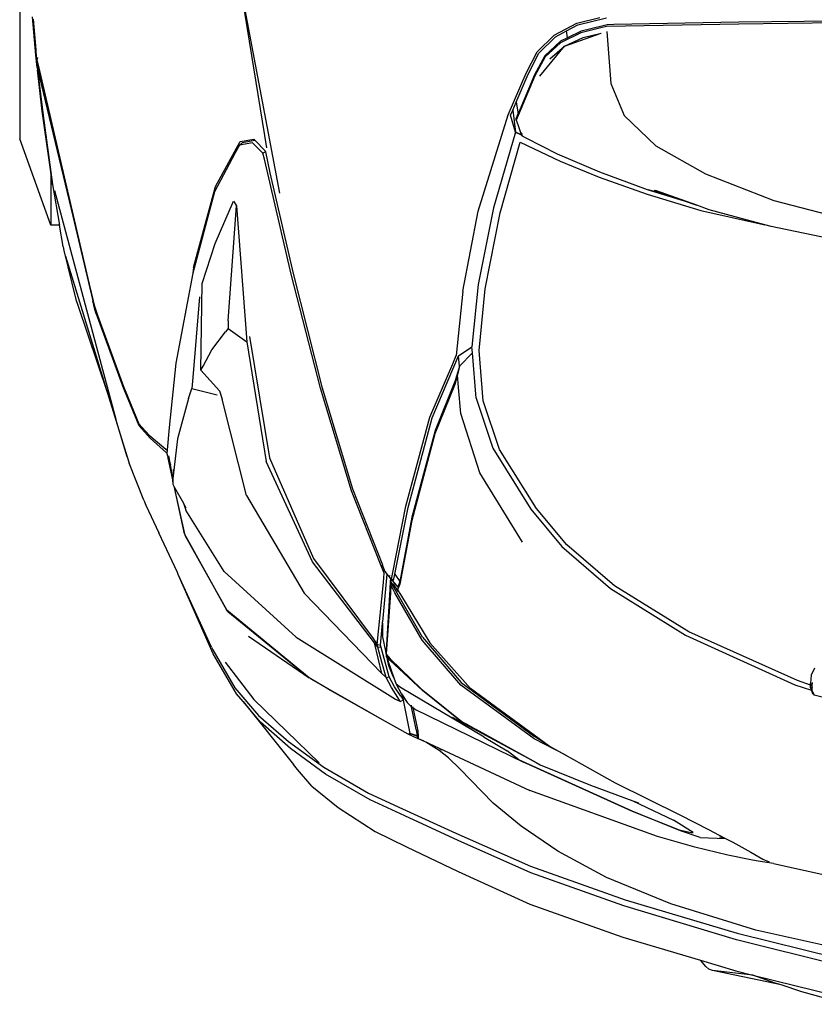
# Model space of a CAD drawing. Units: inches. Extents: x -4737294 to -4736756, y 1716389 to 1717040.
# Tile 3 of 25: x -4737188 to -4737168, y 1716466 to 1716491. Entities that reach past the tile are written whole.
import ezdxf

# ---------------------------------------------------------------- set-up
doc = ezdxf.new("R2010")
doc.units = ezdxf.units.IN
doc.header["$MEASUREMENT"] = 0
doc.layers.add('A-EQPM-VEHI', color=250, linetype='Continuous', lineweight=13)
doc.layers.add('Edges', color=250, linetype='Continuous')

# ---------------------------------------------------------------- blocks, each defined once
blk = doc.blocks.new('Nissan Qashqai pl')
at = {"layer": 'Edges'}
for p, q in [((11.05947, 11.55994), (11.06074, 11.45082)), ((11.06059, 11.56009), (11.06182, 11.4509)), ((11.6016, 11.52761), (11.58664, 11.46068)), ((11.58843, 11.44985), (11.60765, 11.5276)), ((11.61178, 11.52762), (11.59225, 11.44945)), ((11.61272, 11.45895), (11.62966, 11.52759)), ((11.16395, 11.47112), (11.17758, 11.52307)), ((11.45032, 11.49453), (11.45676, 11.51971)), ((11.18773, 11.51111), (11.17906, 11.46956)), ((11.54814, 11.47101), (11.55707, 11.51104)), ((11.62771, 11.50627), (11.62241, 11.48743)), ((11.435, 11.49469), (11.43896, 11.49272)), ((11.44507, 11.49341), (11.44316, 11.49351)), ((11.44373, 11.49245), (11.44491, 11.49291)), ((11.44453, 11.48334), (11.44778, 11.49299)), ((11.44491, 11.49291), (11.44474, 11.49242)), ((11.44507, 11.49341), (11.44491, 11.49291)), ((11.44491, 11.49291), (11.44606, 11.49335)), ((11.44606, 11.49335), (11.44507, 11.49341)), ((11.44786, 11.49325), (11.44606, 11.49335)), ((11.44786, 11.49325), (11.4462, 11.49239)), ((11.44778, 11.49299), (11.4462, 11.49239)), ((11.45018, 11.49392), (11.44778, 11.49299)), ((11.44794, 11.49325), (11.44786, 11.49325)), ((11.45032, 11.49453), (11.44794, 11.49325)), ((11.45018, 11.49392), (11.45032, 11.49453)), ((11.43896, 11.49272), (11.44373, 11.49245)), ((11.44474, 11.49242), (11.44218, 11.48476)), ((11.44474, 11.49242), (11.44373, 11.49245)), ((11.4462, 11.49239), (11.44474, 11.49242)), ((11.62241, 11.48743), (11.61848, 11.47528)), ((11.44218, 11.48476), (11.41383, 11.42186)), ((11.41588, 11.41997), (11.44453, 11.48334)), ((11.14869, 11.43161), (11.16395, 11.47112)), ((11.54814, 11.47101), (11.54666, 11.46197)), ((11.61848, 11.47528), (11.61008, 11.43562)), ((11.61742, 11.47198), (11.61272, 11.45895)), ((11.61848, 11.47528), (11.61742, 11.47198)), ((11.17808, 11.46592), (11.1694, 11.43374)), ((11.1699, 11.42889), (11.17797, 11.4652)), ((11.17797, 11.4652), (11.17808, 11.46592)), ((11.17906, 11.46956), (11.17808, 11.46592)), ((11.54162, 11.45783), (11.54554, 11.46484)), ((11.54554, 11.46484), (11.54721, 11.46841)), ((11.54611, 11.45874), (11.54336, 11.44449)), ((11.54666, 11.46197), (11.54611, 11.45874)), ((11.58664, 11.46068), (11.57152, 11.41151)), ((11.61272, 11.45895), (11.61008, 11.43562)), ((11.61028, 11.44915), (11.61272, 11.45895)), ((11.53572, 11.44731), (11.54162, 11.45783)), ((11.06074, 11.45082), (11.06214, 11.37845)), ((11.06182, 11.4509), (11.06324, 11.37414)), ((11.53354, 11.44315), (11.53572, 11.44731)), ((11.56912, 11.38501), (11.58843, 11.44985)), ((11.59225, 11.44945), (11.57263, 11.38419)), ((11.60419, 11.42861), (11.61028, 11.44915)), ((11.52833, 11.43321), (11.53335, 11.4428)), ((11.53261, 11.43965), (11.5333, 11.44225)), ((11.53313, 11.42848), (11.53354, 11.44315)), ((11.5333, 11.44225), (11.53335, 11.4428)), ((11.53335, 11.4428), (11.53354, 11.44315)), ((11.54336, 11.44449), (11.53855, 11.42543)), ((11.1323, 11.40268), (11.14869, 11.43161)), ((11.1694, 11.43374), (11.1668, 11.42651)), ((11.5202, 11.41712), (11.52833, 11.43321)), ((11.60772, 11.43162), (11.60419, 11.42861)), ((11.60938, 11.43347), (11.60772, 11.43162)), ((11.61008, 11.43562), (11.60938, 11.43347)), ((11.1668, 11.42651), (11.1582, 11.40259)), ((11.16047, 11.39766), (11.1699, 11.42889)), ((11.16426, 11.41918), (11.1668, 11.42651)), ((11.53313, 11.42848), (11.52922, 11.417)), ((11.53855, 11.42543), (11.53253, 11.4038)), ((11.59084, 11.38361), (11.60419, 11.42861)), ((11.15764, 11.39828), (11.16426, 11.41918)), ((11.15766, 11.39771), (11.16426, 11.41918)), ((11.16426, 11.41918), (11.15826, 11.40186)), ((11.41383, 11.42186), (11.38718, 11.37878)), ((11.38877, 11.37638), (11.41588, 11.41997)), ((11.53009, 11.42439), (11.52299, 11.41307)), ((11.52855, 11.41625), (11.53022, 11.42324)), ((11.53022, 11.42324), (11.53009, 11.42439)), ((11.50131, 11.37908), (11.5202, 11.41712)), ((11.5118, 11.38938), (11.52299, 11.41307)), ((11.52922, 11.417), (11.51787, 11.38901)), ((11.51787, 11.38901), (11.52855, 11.41625)), ((11.57152, 11.41151), (11.55624, 11.37411)), ((11.11477, 11.38434), (11.1323, 11.40268)), ((11.53253, 11.4038), (11.50574, 11.32965)), ((11.14751, 11.37001), (11.15766, 11.39771)), ((11.15051, 11.36998), (11.16047, 11.39766)), ((11.5118, 11.38938), (11.51304, 11.39274)), ((11.51787, 11.38901), (11.48801, 11.32337)), ((11.49005, 11.3275), (11.51787, 11.38901)), ((11.50277, 11.36495), (11.5118, 11.38938)), ((11.54963, 11.33002), (11.56912, 11.38501)), ((11.09618, 11.37663), (11.11477, 11.38434)), ((11.48518, 11.35017), (11.50131, 11.37908)), ((11.57263, 11.38419), (11.5535, 11.33028)), ((11.57164, 11.32969), (11.59084, 11.38361)), ((11.06236, 11.3576), (11.05822, 11.37418)), ((11.06214, 11.37845), (11.06222, 11.37449)), ((11.06222, 11.37449), (11.06303, 11.37135)), ((11.06324, 11.37414), (11.06408, 11.37085)), ((11.06624, 11.37435), (11.09618, 11.37663)), ((11.38718, 11.37878), (11.3635, 11.35125)), ((11.36451, 11.34835), (11.38877, 11.37638)), ((11.55624, 11.37411), (11.54097, 11.34593)), ((11.06139, 11.35691), (11.05807, 11.37037)), ((11.06303, 11.37135), (11.06594, 11.3594)), ((11.06408, 11.37085), (11.06692, 11.35921)), ((11.06961, 11.36056), (11.0671, 11.37109)), ((11.07472, 11.34981), (11.0671, 11.37109)), ((11.13692, 11.34555), (11.14751, 11.37001)), ((11.14123, 11.34726), (11.15051, 11.36998)), ((11.49086, 11.33567), (11.50277, 11.36495)), ((11.06818, 11.34377), (11.06139, 11.35691)), ((11.06584, 11.35092), (11.06236, 11.3576)), ((11.06594, 11.3594), (11.06978, 11.35164)), ((11.06692, 11.35921), (11.0727, 11.34754)), ((11.07472, 11.34981), (11.06961, 11.36056)), ((11.06978, 11.35164), (11.06584, 11.35092)), ((11.06918, 11.34452), (11.06584, 11.35092)), ((11.06978, 11.35164), (11.07183, 11.3475)), ((11.3635, 11.35125), (11.34251, 11.3336)), ((11.07183, 11.3475), (11.08018, 11.33842)), ((11.0727, 11.34754), (11.0809, 11.33858)), ((11.08206, 11.34125), (11.07472, 11.34981)), ((11.092, 11.33548), (11.07472, 11.34981)), ((11.12767, 11.32749), (11.13692, 11.34555)), ((11.13017, 11.32416), (11.14123, 11.34726)), ((11.34283, 11.33026), (11.36451, 11.34835)), ((11.48518, 11.35017), (11.4758, 11.33232)), ((11.48012, 11.34111), (11.48518, 11.35017)), ((11.54097, 11.34593), (11.52646, 11.32473)), ((11.07787, 11.3339), (11.06818, 11.34377)), ((11.07866, 11.33492), (11.06918, 11.34452)), ((11.48005, 11.341), (11.44669, 11.29536)), ((11.47876, 11.33901), (11.47454, 11.33252)), ((11.47876, 11.33901), (11.48005, 11.341)), ((11.48005, 11.341), (11.48012, 11.34111)), ((11.09022, 11.32753), (11.07787, 11.3339)), ((11.09081, 11.32882), (11.07866, 11.33492)), ((11.08018, 11.33842), (11.09121, 11.33249)), ((11.0809, 11.33858), (11.09174, 11.33271)), ((11.34251, 11.3336), (11.3082, 11.31215)), ((11.46332, 11.28473), (11.48966, 11.33337)), ((11.47038, 11.29841), (11.49086, 11.33567)), ((11.47038, 11.29841), (11.48966, 11.33337)), ((11.48966, 11.33337), (11.49086, 11.33567)), ((11.11439, 11.31711), (11.09022, 11.32753)), ((11.10704, 11.32181), (11.09081, 11.32882)), ((11.09121, 11.33249), (11.1138, 11.3229)), ((11.09174, 11.33271), (11.11486, 11.323)), ((11.12645, 11.32495), (11.12767, 11.32749)), ((11.30757, 11.30833), (11.34283, 11.33026)), ((11.44331, 11.28988), (11.47454, 11.33252)), ((11.4758, 11.33232), (11.44474, 11.28965)), ((11.48133, 11.27727), (11.50574, 11.32965)), ((11.48983, 11.32694), (11.49005, 11.3275)), ((11.53062, 11.28691), (11.54963, 11.33002)), ((11.5535, 11.33028), (11.53487, 11.28826)), ((11.55274, 11.28821), (11.57164, 11.32969)), ((11.10704, 11.32181), (11.1138, 11.3229)), ((11.11164, 11.31982), (11.10704, 11.32181)), ((11.1138, 11.3229), (11.11393, 11.32284)), ((11.11393, 11.32284), (11.1164, 11.32172)), ((11.11486, 11.323), (11.1172, 11.32196)), ((11.1164, 11.32172), (11.1172, 11.32196)), ((11.11744, 11.32189), (11.1164, 11.32172)), ((11.1172, 11.32196), (11.11744, 11.32189)), ((11.11744, 11.32189), (11.11997, 11.32267)), ((11.11997, 11.32267), (11.12459, 11.32429)), ((11.12604, 11.32481), (11.1244, 11.32146)), ((11.1244, 11.32146), (11.12591, 11.32476)), ((11.12459, 11.32429), (11.12591, 11.32476)), ((11.12466, 11.32442), (11.12595, 11.32486)), ((11.12478, 11.32467), (11.12595, 11.32486)), ((11.12595, 11.32486), (11.1251, 11.3253)), ((11.12591, 11.32476), (11.12595, 11.32486)), ((11.12591, 11.32476), (11.12604, 11.32481)), ((11.12595, 11.32486), (11.12626, 11.32554)), ((11.12595, 11.32486), (11.12607, 11.32488)), ((11.12604, 11.32481), (11.12645, 11.32495)), ((11.12607, 11.32488), (11.12604, 11.32481)), ((11.12631, 11.32537), (11.12607, 11.32488)), ((11.12607, 11.32488), (11.12645, 11.32495)), ((11.17121, 11.31245), (11.13017, 11.32416)), ((11.36192, 11.32544), (11.32179, 11.30083)), ((11.45883, 11.26345), (11.48954, 11.32636)), ((11.48801, 11.32337), (11.48281, 11.31653)), ((11.48983, 11.32694), (11.48954, 11.32636)), ((11.52646, 11.32473), (11.51313, 11.30854)), ((11.11164, 11.31982), (11.1244, 11.32146)), ((11.11467, 11.31851), (11.11164, 11.31982)), ((11.17021, 11.29978), (11.11439, 11.31711)), ((11.1244, 11.32146), (11.11467, 11.31851)), ((11.1244, 11.32146), (11.16836, 11.30873)), ((11.47499, 11.30324), (11.48281, 11.31653)), ((11.21523, 11.3038), (11.17121, 11.31245)), ((11.3082, 11.31215), (11.28005, 11.30276)), ((11.16836, 11.30873), (11.21271, 11.29983)), ((11.27848, 11.29865), (11.30757, 11.30833)), ((11.51313, 11.30854), (11.49329, 11.28912)), ((11.21656, 11.2908), (11.17021, 11.29978)), ((11.21271, 11.29983), (11.24875, 11.29618)), ((11.2509, 11.3003), (11.21523, 11.3038)), ((11.28005, 11.30276), (11.2509, 11.3003)), ((11.32179, 11.30083), (11.28736, 11.28974)), ((11.47499, 11.30324), (11.4462, 11.25482)), ((11.25238, 11.29648), (11.24875, 11.29618)), ((11.2541, 11.28846), (11.24875, 11.29618)), ((11.27848, 11.29865), (11.25238, 11.29648)), ((11.25238, 11.29648), (11.25993, 11.28891)), ((11.42028, 11.27173), (11.44669, 11.29536)), ((11.46746, 11.29312), (11.47026, 11.29821)), ((11.47026, 11.29821), (11.47038, 11.29841)), ((11.21656, 11.2908), (11.25377, 11.28706)), ((11.25993, 11.28891), (11.2541, 11.28846)), ((11.29, 11.2731), (11.2541, 11.28846)), ((11.25993, 11.28891), (11.25999, 11.28889)), ((11.25999, 11.28889), (11.26503, 11.28789)), ((11.25999, 11.28889), (11.26771, 11.28668)), ((11.27242, 11.28847), (11.26503, 11.28789)), ((11.26503, 11.28789), (11.27055, 11.28622)), ((11.28736, 11.28974), (11.27242, 11.28847)), ((11.41708, 11.26758), (11.44331, 11.28988)), ((11.44474, 11.28965), (11.41866, 11.26734)), ((11.44691, 11.26684), (11.46587, 11.29022)), ((11.46538, 11.28932), (11.44788, 11.2676)), ((11.46538, 11.28932), (11.46587, 11.29022)), ((11.46587, 11.29022), (11.46737, 11.29293)), ((11.46746, 11.29312), (11.46737, 11.29293)), ((11.49329, 11.28912), (11.48692, 11.28262)), ((11.53487, 11.28826), (11.52058, 11.25724)), ((11.53843, 11.2583), (11.55274, 11.28821)), ((11.25857, 11.28503), (11.25377, 11.28706)), ((11.28951, 11.27177), (11.25857, 11.28503)), ((11.26771, 11.28668), (11.26785, 11.28663)), ((11.26785, 11.28663), (11.29721, 11.27493)), ((11.27055, 11.28622), (11.29928, 11.27468)), ((11.48692, 11.28262), (11.48256, 11.27724)), ((11.51652, 11.25601), (11.53062, 11.28691)), ((11.47707, 11.26812), (11.48133, 11.27727)), ((11.48256, 11.27724), (11.47783, 11.26953)), ((11.48133, 11.27727), (11.48217, 11.27864)), ((11.3411, 11.25789), (11.28951, 11.27177)), ((11.34188, 11.25916), (11.29, 11.2731)), ((11.29721, 11.27493), (11.34742, 11.26142)), ((11.29928, 11.27468), (11.34932, 11.2614)), ((11.39234, 11.25471), (11.42028, 11.27173)), ((11.41708, 11.26758), (11.38507, 11.24911)), ((11.41866, 11.26734), (11.3914, 11.25156)), ((11.42958, 11.2488), (11.44691, 11.26684)), ((11.44788, 11.2676), (11.43028, 11.24852)), ((11.46049, 11.26254), (11.47129, 11.26473)), ((11.47129, 11.26473), (11.47442, 11.26498)), ((11.47585, 11.26509), (11.47322, 11.2592)), ((11.47442, 11.26498), (11.47433, 11.26475)), ((11.47442, 11.26498), (11.47446, 11.26498)), ((11.47445, 11.26477), (11.47446, 11.26498)), ((11.47446, 11.26498), (11.47482, 11.26501)), ((11.47585, 11.26509), (11.47463, 11.26457)), ((11.47482, 11.26501), (11.47475, 11.26484)), ((11.47482, 11.26501), (11.47585, 11.26509)), ((11.47588, 11.26517), (11.47585, 11.26509)), ((11.47783, 11.26953), (11.47588, 11.26517)), ((11.47707, 11.26812), (11.47588, 11.26517)), ((11.38043, 11.25154), (11.34188, 11.25916)), ((11.34742, 11.26142), (11.38475, 11.2543)), ((11.34932, 11.2614), (11.38634, 11.25437)), ((11.47278, 11.2604), (11.45351, 11.25651)), ((11.45491, 11.25868), (11.45678, 11.26054)), ((11.4564, 11.26086), (11.45669, 11.26088)), ((11.45652, 11.26104), (11.45688, 11.26111)), ((11.45678, 11.26054), (11.45714, 11.2609)), ((11.45714, 11.2609), (11.45732, 11.2612)), ((11.45729, 11.26188), (11.45734, 11.2619)), ((11.47041, 11.26385), (11.45732, 11.2612)), ((11.45732, 11.2612), (11.45781, 11.262)), ((11.45736, 11.26195), (11.45734, 11.2619)), ((11.45736, 11.26195), (11.45755, 11.26195)), ((11.45781, 11.262), (11.45883, 11.26345)), ((11.45781, 11.262), (11.46047, 11.26254)), ((11.46047, 11.26254), (11.46049, 11.26254)), ((11.47322, 11.2592), (11.46579, 11.24614)), ((11.47041, 11.26385), (11.47423, 11.26446)), ((11.47269, 11.26007), (11.47281, 11.2603)), ((11.47463, 11.26457), (11.47278, 11.2604)), ((11.47423, 11.26446), (11.47278, 11.2604)), ((11.47278, 11.2604), (11.47281, 11.2603)), ((11.47281, 11.2603), (11.47317, 11.26096)), ((11.47281, 11.2603), (11.47322, 11.2592)), ((11.47423, 11.26446), (11.47445, 11.26449)), ((11.47463, 11.26457), (11.47445, 11.26449)), ((11.37955, 11.25028), (11.3411, 11.25789)), ((11.38043, 11.25154), (11.38475, 11.2543)), ((11.38475, 11.2543), (11.38801, 11.25321)), ((11.38634, 11.25437), (11.38953, 11.25299)), ((11.39063, 11.25338), (11.38862, 11.25223)), ((11.38953, 11.25299), (11.39234, 11.25471)), ((11.44418, 11.2522), (11.44968, 11.25519)), ((11.4462, 11.25482), (11.44418, 11.2522)), ((11.45121, 11.25489), (11.44573, 11.25131)), ((11.44968, 11.25519), (11.44984, 11.25529)), ((11.44984, 11.25529), (11.45491, 11.25868)), ((11.44984, 11.25529), (11.45351, 11.25651)), ((11.45121, 11.25489), (11.45351, 11.25651)), ((11.45386, 11.25448), (11.45199, 11.25317)), ((11.45295, 11.25195), (11.45421, 11.25473)), ((11.45316, 11.25595), (11.45351, 11.25651)), ((11.45351, 11.25651), (11.45421, 11.25473)), ((11.45421, 11.25473), (11.45386, 11.25448)), ((11.47197, 11.25711), (11.47177, 11.25676)), ((11.50736, 11.23616), (11.51652, 11.25601)), ((11.52058, 11.25724), (11.51126, 11.23721)), ((11.52949, 11.24004), (11.53843, 11.2583)), ((11.38338, 11.24949), (11.37955, 11.25028)), ((11.38041, 11.24692), (11.38275, 11.24887)), ((11.38408, 11.25081), (11.38043, 11.25154)), ((11.38129, 11.24847), (11.38167, 11.2488)), ((11.38275, 11.24887), (11.38338, 11.24949)), ((11.38295, 11.24897), (11.38801, 11.25321)), ((11.38446, 11.24984), (11.38295, 11.24897)), ((11.38295, 11.24897), (11.38491, 11.2491)), ((11.38295, 11.24897), (11.38461, 11.24885)), ((11.38408, 11.25081), (11.38338, 11.24949)), ((11.38461, 11.24885), (11.38464, 11.24887)), ((11.38461, 11.24885), (11.38934, 11.2486)), ((11.38464, 11.24887), (11.38501, 11.24911)), ((11.38491, 11.2491), (11.38464, 11.24887)), ((11.38823, 11.2519), (11.38491, 11.2491)), ((11.38501, 11.24911), (11.38507, 11.24911)), ((11.38507, 11.24911), (11.3867, 11.24922)), ((11.38811, 11.25194), (11.3861, 11.25078)), ((11.3914, 11.25156), (11.3867, 11.24922)), ((11.3867, 11.24922), (11.3915, 11.24906)), ((11.38862, 11.25223), (11.38822, 11.252)), ((11.38862, 11.25223), (11.38823, 11.2519)), ((11.38953, 11.25299), (11.38862, 11.25223)), ((11.38934, 11.2486), (11.42481, 11.24653)), ((11.3915, 11.24906), (11.42659, 11.2465)), ((11.41698, 11.19425), (11.45295, 11.25195)), ((11.43996, 11.24823), (11.42296, 11.24352)), ((11.42684, 11.24649), (11.42958, 11.2488)), ((11.43028, 11.24852), (11.42784, 11.24647)), ((11.42996, 11.24721), (11.43609, 11.24937)), ((11.43368, 11.248), (11.42996, 11.24721)), ((11.4397, 11.25049), (11.43368, 11.248)), ((11.43609, 11.24937), (11.44061, 11.25095)), ((11.44061, 11.25095), (11.4397, 11.25049)), ((11.44573, 11.25131), (11.43996, 11.24823)), ((11.44027, 11.24637), (11.43996, 11.24823)), ((11.44624, 11.24948), (11.44027, 11.24637)), ((11.44061, 11.25095), (11.44418, 11.2522)), ((11.45199, 11.25317), (11.44624, 11.24948)), ((11.33108, 11.22699), (11.37506, 11.24429)), ((11.37475, 11.24309), (11.33228, 11.22637)), ((11.38, 11.24532), (11.37475, 11.24309)), ((11.37506, 11.24429), (11.37524, 11.24436)), ((11.37506, 11.24429), (11.37621, 11.24429)), ((11.37922, 11.24593), (11.37524, 11.24436)), ((11.3763, 11.24436), (11.37524, 11.24436)), ((11.37922, 11.24593), (11.38041, 11.24692)), ((11.37933, 11.24631), (11.37922, 11.24593)), ((11.38533, 11.24487), (11.38, 11.24532)), ((11.38041, 11.24692), (11.40818, 11.24436)), ((11.42115, 11.24117), (11.38533, 11.24487)), ((11.3915, 11.19885), (11.4381, 11.24397)), ((11.41644, 11.24436), (11.40818, 11.24436)), ((11.40898, 11.24429), (11.40818, 11.24436)), ((11.40898, 11.24429), (11.4163, 11.24429)), ((11.4152, 11.24371), (11.40898, 11.24429)), ((11.4163, 11.24429), (11.4152, 11.24371)), ((11.42154, 11.24313), (11.4152, 11.24371)), ((11.41644, 11.24436), (11.4163, 11.24429)), ((11.41686, 11.24458), (11.41644, 11.24436)), ((11.4252, 11.2462), (11.41686, 11.24458)), ((11.42115, 11.24117), (11.42154, 11.24313)), ((11.42296, 11.24352), (11.42154, 11.24313)), ((11.43154, 11.24397), (11.42287, 11.24164)), ((11.42296, 11.24352), (11.42287, 11.24164)), ((11.42481, 11.24653), (11.42659, 11.2465)), ((11.42659, 11.2465), (11.4252, 11.2462)), ((11.42659, 11.2465), (11.42684, 11.24649)), ((11.42684, 11.24649), (11.42784, 11.24647)), ((11.42784, 11.24647), (11.42996, 11.24721)), ((11.4381, 11.24397), (11.42915, 11.24177)), ((11.44027, 11.24637), (11.43154, 11.24397)), ((11.4381, 11.24397), (11.44027, 11.24637)), ((11.44114, 11.20281), (11.46562, 11.24583)), ((11.44697, 11.21272), (11.46562, 11.24583)), ((11.46562, 11.24583), (11.46579, 11.24614)), ((11.3715, 11.20434), (11.41772, 11.23895)), ((11.42033, 11.23975), (11.37334, 11.20375)), ((11.41772, 11.23895), (11.41931, 11.23998)), ((11.41915, 11.23969), (11.4194, 11.23996)), ((11.41931, 11.23998), (11.4196, 11.24017)), ((11.4194, 11.23996), (11.41931, 11.23998)), ((11.4194, 11.23996), (11.4196, 11.24017)), ((11.41958, 11.23992), (11.4194, 11.23996)), ((11.4196, 11.24017), (11.42014, 11.24052)), ((11.41984, 11.24006), (11.42014, 11.24052)), ((11.42014, 11.24052), (11.42115, 11.24117)), ((11.42915, 11.24177), (11.42033, 11.23975)), ((11.42287, 11.24164), (11.42033, 11.23975)), ((11.42178, 11.24134), (11.42115, 11.24117)), ((11.42287, 11.24164), (11.42178, 11.24134)), ((11.42216, 11.24127), (11.42178, 11.24134)), ((11.51126, 11.23721), (11.49628, 11.21137)), ((11.51576, 11.21859), (11.52949, 11.24004)), ((11.49236, 11.21027), (11.50736, 11.23616)), ((11.27199, 11.20923), (11.33108, 11.22699)), ((11.33228, 11.22637), (11.27276, 11.20843)), ((11.50327, 11.20341), (11.51576, 11.21859)), ((11.20627, 11.19262), (11.27199, 11.20923)), ((11.27276, 11.20843), (11.20665, 11.19145)), ((11.44697, 11.21272), (11.44114, 11.20281)), ((11.47745, 11.18983), (11.49236, 11.21027)), ((11.49628, 11.21137), (11.48154, 11.19102)), ((11.31316, 11.17892), (11.3715, 11.20434)), ((11.37334, 11.20375), (11.31527, 11.17691)), ((11.44081, 11.20225), (11.44046, 11.20182)), ((11.4411, 11.20277), (11.44081, 11.20225)), ((11.44114, 11.20281), (11.4411, 11.20277)), ((11.45306, 11.16974), (11.48975, 11.20767)), ((11.50327, 11.20341), (11.49363, 11.19502)), ((11.33497, 11.16556), (11.3915, 11.19885)), ((11.44046, 11.20182), (11.40144, 11.15414)), ((11.40216, 11.15476), (11.44046, 11.20182)), ((11.41633, 11.16662), (11.44046, 11.20182)), ((11.20665, 11.19145), (11.14012, 11.17593)), ((11.14803, 11.17913), (11.20627, 11.19262)), ((11.37896, 11.15265), (11.41698, 11.19425)), ((11.45433, 11.16358), (11.49082, 11.19282)), ((11.48154, 11.19102), (11.46617, 11.17358)), ((11.49363, 11.19502), (11.49082, 11.19282)), ((11.46237, 11.17248), (11.47745, 11.18983)), ((11.03575, 11.16129), (11.1598, 11.18473)), ((11.04919, 11.16347), (11.13359, 11.17719)), ((11.12929, 11.17052), (11.13526, 11.17642)), ((11.13658, 11.17502), (11.1347, 11.17313)), ((11.13526, 11.17642), (11.13585, 11.17654)), ((11.13585, 11.17654), (11.14803, 11.17913)), ((11.13585, 11.17654), (11.13658, 11.17502)), ((11.14012, 11.17593), (11.13658, 11.17502)), ((11.24278, 11.16729), (11.31316, 11.17892)), ((11.24587, 11.16563), (11.31527, 11.17691)), ((11.46617, 11.17358), (11.45433, 11.16358)), ((11.12846, 11.16971), (11.12929, 11.17052)), ((11.12977, 11.16183), (11.12846, 11.16971)), ((11.12929, 11.17052), (11.13057, 11.16299)), ((11.1347, 11.17313), (11.13062, 11.16899)), ((11.13062, 11.16899), (11.13192, 11.16144)), ((11.43143, 11.15309), (11.45306, 11.16974)), ((11.44642, 11.15882), (11.46237, 11.17248)), ((11.13192, 11.16144), (11.13057, 11.16299)), ((11.16717, 11.15976), (11.24587, 11.16563)), ((11.23823, 11.15494), (11.24587, 11.16563)), ((11.33497, 11.16556), (11.27913, 11.15147)), ((11.45433, 11.16358), (11.44983, 11.15977)), ((11.15597, 11.14759), (11.12977, 11.16183)), ((11.13192, 11.16144), (11.13652, 11.15905)), ((11.13652, 11.15905), (11.15893, 11.14704)), ((11.16444, 11.15792), (11.16717, 11.15976)), ((11.18896, 11.14734), (11.16444, 11.15792)), ((11.23369, 11.15498), (11.16717, 11.15976)), ((11.42433, 11.14593), (11.44642, 11.15882)), ((11.44983, 11.15977), (11.42671, 11.14629)), ((11.23369, 11.15498), (11.23823, 11.15494)), ((11.23823, 11.15494), (11.2401, 11.15337)), ((11.25046, 11.1455), (11.2401, 11.15337)), ((11.27429, 11.14993), (11.27913, 11.15147)), ((11.37896, 11.15265), (11.34336, 11.13032)), ((11.40144, 11.15414), (11.3571, 11.12956)), ((11.35832, 11.12998), (11.40144, 11.15414)), ((11.40216, 11.15476), (11.40144, 11.15414)), ((11.20291, 11.13489), (11.15597, 11.14759)), ((11.15893, 11.14704), (11.20616, 11.13437)), ((11.2121, 11.1399), (11.18896, 11.14734)), ((11.26005, 11.1405), (11.25046, 11.1455)), ((11.27429, 11.14993), (11.26224, 11.13901)), ((11.27289, 11.13379), (11.27664, 11.14845)), ((11.42671, 11.14629), (11.38067, 11.12595)), ((11.42283, 11.14525), (11.38067, 11.12595)), ((11.42283, 11.14525), (11.42433, 11.14593)), ((11.26224, 11.13901), (11.2121, 11.1399)), ((11.26224, 11.13901), (11.26005, 11.1405)), ((11.20291, 11.13489), (11.20295, 11.13488)), ((11.20295, 11.13488), (11.20616, 11.13437)), ((11.20616, 11.13437), (11.25827, 11.12461)), ((11.21991, 11.1382), (11.26663, 11.13449)), ((11.26663, 11.13449), (11.27289, 11.13379)), ((11.27871, 11.13184), (11.27289, 11.13379)), ((11.27871, 11.13184), (11.30218, 11.1256)), ((11.32955, 11.12347), (11.3571, 11.12956)), ((11.3571, 11.12956), (11.33021, 11.12384)), ((11.33021, 11.12384), (11.33938, 11.12898)), ((11.33938, 11.12898), (11.34202, 11.13045)), ((11.33938, 11.12898), (11.34336, 11.13032)), ((11.3571, 11.12956), (11.35832, 11.12998)), ((11.25827, 11.12461), (11.29558, 11.12077)), ((11.30218, 11.1256), (11.32517, 11.12286)), ((11.31323, 11.11986), (11.32588, 11.12266)), ((11.32423, 11.12258), (11.314, 11.12039)), ((11.32423, 11.12258), (11.31704, 11.12142)), ((11.31982, 11.1231), (11.32517, 11.12286)), ((11.32423, 11.12258), (11.32588, 11.12266)), ((11.32517, 11.12286), (11.32831, 11.12278)), ((11.32588, 11.12266), (11.32831, 11.12278)), ((11.32831, 11.12278), (11.32955, 11.12347)), ((11.32955, 11.12347), (11.33021, 11.12384)), ((11.37962, 11.12547), (11.35656, 11.11477)), ((11.38067, 11.12595), (11.37962, 11.12547)), ((11.29558, 11.12077), (11.30849, 11.1195)), ((11.30003, 11.10916), (11.30813, 11.11883)), ((11.31027, 11.11923), (11.30178, 11.10961)), ((11.30805, 11.11884), (11.30863, 11.11948)), ((11.30813, 11.11883), (11.30863, 11.11948)), ((11.30849, 11.1195), (11.30863, 11.11948)), ((11.30863, 11.11948), (11.31033, 11.1193)), ((11.31033, 11.1193), (11.31027, 11.11923)), ((11.31033, 11.1193), (11.31061, 11.11927)), ((11.31061, 11.11927), (11.314, 11.12039)), ((11.31704, 11.12142), (11.31186, 11.12058)), ((11.314, 11.12039), (11.31704, 11.12142)), ((11.34052, 11.10725), (11.35656, 11.11477)), ((11.29339, 11.10313), (11.30003, 11.10916)), ((11.30178, 11.10961), (11.29459, 11.10327)), ((11.33757, 11.10603), (11.31612, 11.09747)), ((11.33757, 11.10603), (11.34052, 11.10725)), ((11.29459, 11.10327), (11.27358, 11.0947)), ((11.27407, 11.09522), (11.29339, 11.10313)), ((11.2732, 11.09452), (11.22772, 11.07792)), ((11.23038, 11.07923), (11.27187, 11.09432)), ((11.27187, 11.09432), (11.27407, 11.09522)), ((11.27358, 11.0947), (11.2732, 11.09452)), ((11.27358, 11.0947), (11.27407, 11.09522)), ((11.27568, 11.08503), (11.31244, 11.09628)), ((11.31244, 11.09628), (11.29065, 11.08989)), ((11.30801, 11.09508), (11.30877, 11.09528)), ((11.31244, 11.09628), (11.31612, 11.09747)), ((11.15816, 11.05423), (11.29065, 11.08989)), ((11.19633, 11.06072), (11.27568, 11.08503)), ((11.22475, 11.06772), (11.27568, 11.08503)), ((11.22216, 11.0766), (11.08821, 11.045)), ((11.09177, 11.04531), (11.22216, 11.0766)), ((11.21998, 11.07614), (11.22216, 11.0766)), ((11.2222, 11.07656), (11.22216, 11.0766)), ((11.22715, 11.07771), (11.2222, 11.07656)), ((11.22238, 11.07665), (11.2222, 11.07656)), ((11.22238, 11.07665), (11.22532, 11.07737)), ((11.22532, 11.07737), (11.23038, 11.07923)), ((11.22731, 11.07783), (11.22706, 11.07777)), ((11.22962, 11.07837), (11.22715, 11.07771)), ((11.22772, 11.07792), (11.22715, 11.07771)), ((11.22962, 11.07837), (11.22772, 11.07792)), ((11.08649, 11.04496), (11.21998, 11.07614)), ((11.19297, 11.05964), (11.22148, 11.06662)), ((11.22148, 11.06662), (11.22475, 11.06772)), ((11.19089, 11.05929), (11.19297, 11.05964)), ((11.15472, 11.05317), (11.17828, 11.05716)), ((11.19065, 11.05923), (11.17828, 11.05716)), ((11.17828, 11.05716), (11.17828, 11.05208)), ((11.19089, 11.05929), (11.19065, 11.05923)), ((11.14751, 11.05208), (11.11234, 11.04716)), ((11.11474, 11.04762), (11.15472, 11.05317)), ((11.17828, 11.05208), (11.12828, 11.03408)), ((11.15248, 11.05278), (11.14751, 11.05208)), ((11.14751, 11.05208), (11.17828, 11.05208)), ((11.15472, 11.05317), (11.15248, 11.05278)), ((11.07977, 11.04339), (11.05762, 11.04159)), ((11.05899, 11.04188), (11.07681, 11.04337)), ((11.07681, 11.04337), (11.08106, 11.04371)), ((11.08696, 11.04422), (11.07977, 11.04339)), ((11.08106, 11.04371), (11.08273, 11.0441)), ((11.08114, 11.04436), (11.08208, 11.0442)), ((11.08273, 11.0441), (11.08562, 11.04476)), ((11.08273, 11.0441), (11.08365, 11.04395)), ((11.08821, 11.045), (11.08365, 11.04395)), ((11.08365, 11.04395), (11.08696, 11.04422)), ((11.08562, 11.04476), (11.08649, 11.04496)), ((11.08649, 11.04496), (11.08796, 11.04514)), ((11.08696, 11.04422), (11.08721, 11.04424)), ((11.08728, 11.04426), (11.08721, 11.04424)), ((11.08728, 11.04426), (11.08834, 11.04438)), ((11.08834, 11.04438), (11.11474, 11.04762)), ((11.11234, 11.04716), (11.08834, 11.04438)), ((10.95773, 11.03408), (11.12828, 11.03408))]:
    blk.add_line(p, q, dxfattribs=at)
blk = doc.blocks.new('car')
blk.add_blockref('Nissan Qashqai pl', (-9.74328, -11.91512))

msp = doc.modelspace()

# ---------------------------------------------------------------- block references
at = {"layer": 'A-EQPM-VEHI', "xscale": 43.56002006885659, "yscale": 43.56002006885659, "zscale": 43.56002006885659, "rotation": 270}
msp.add_blockref('car', (-4737150.017, 1716548.61), dxfattribs=at)

doc.saveas('drawing.dxf')
